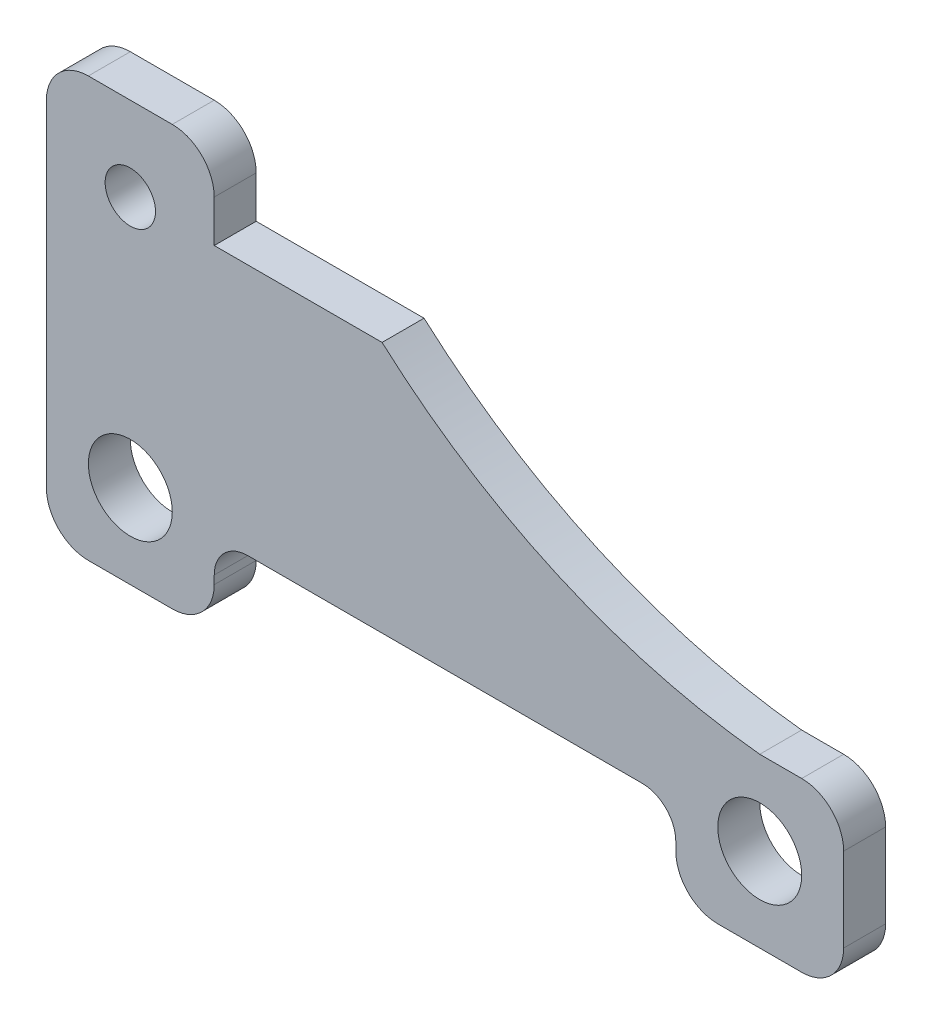
from build123d import *

# Parameters (mm, degrees)
CARRIAGE_PLATE_PROFILE_R   = 5
CARRIAGE_PLATE_PROFILE_R_2 = 3
CARRIAGE_PLATE_5MM_DEPTH   = 5


with BuildPart() as part:
    # Carriage Plate Profile → Carriage Plate 5mm (new body)
    with BuildSketch(Plane.XY):
        with BuildLine():
            Line((-10, -5), (-10, 35))
            ThreePointArc((-10, 35), (-8.535533906, 38.535533906), (-5, 40))
            Line((-5, 40), (5, 40))
            ThreePointArc((5, 40), (8.535533906, 38.535533906), (10, 35))
            Line((10, 35), (10, 30))
            Line((10, 30), (30, 30))
            ThreePointArc((30, 30), (50.922837109, 16.451383494), (75, 10))
            Line((75, 10), (80, 10))
            ThreePointArc((80, 10), (83.535533906, 8.535533906), (85, 5))
            Line((85, 5), (85, -5))
            ThreePointArc((85, -5), (83.535533906, -8.535533906), (80, -10))
            Line((80, -10), (75, -10))
            Line((75, -10), (70, -10))
            ThreePointArc((70, -10), (66.464466094, -8.535533906), (65, -5))
            Line((65, -5), (65, -4))
            ThreePointArc((65, -4), (63.828427125, -1.171572875), (61, 0))
            Line((61, 0), (14, 0))
            ThreePointArc((14, 0), (11.171572875, -1.171572875), (10, -4))
            Line((10, -4), (10, -5))
            ThreePointArc((10, -5), (8.535533906, -8.535533906), (5, -10))
            Line((5, -10), (-5, -10))
            ThreePointArc((-5, -10), (-8.535533906, -8.535533906), (-10, -5))
        make_face()
        Circle(CARRIAGE_PLATE_PROFILE_R, mode=Mode.SUBTRACT)
        with Locations((75, 0)):
            Circle(CARRIAGE_PLATE_PROFILE_R, mode=Mode.SUBTRACT)
        with Locations((0, 30)):
            Circle(CARRIAGE_PLATE_PROFILE_R_2, mode=Mode.SUBTRACT)
    extrude(amount=CARRIAGE_PLATE_5MM_DEPTH)


solid = part.part
